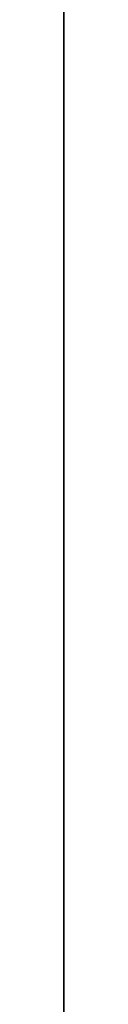
# Model space of a CAD drawing. Units: inches. Extents: x 2083 to 3317, y 1141 to 2115.
# Tile 37 of 256: x 2235.95978 to 2235.95981, y 1477.84234 to 1477.92601. Entities that reach past the tile are written whole.
import ezdxf

# ---------------------------------------------------------------- set-up
doc = ezdxf.new("R2010")
doc.units = ezdxf.units.IN
doc.layers.add('A-ANNO-DIMS', color=2, linetype='Continuous', lineweight=18)
doc.layers.add('A-WALL', color=7, linetype='Continuous', lineweight=35)
doc.layers.add('A-WALL-PATT', color=251, linetype='Continuous', lineweight=13, true_color=0x636466)
doc.styles.get("Standard").update_dxf_attribs({"font": 'arial.ttf'})
doc.dimstyles.new('ISO-25', dxfattribs={"dimtxt": 12, "dimasz": 12, "dimexe": 1.25, "dimexo": 0.625, "dimtad": 1, "dimlunit": 3, "dimtxsty": 'Standard', "dimcen": 2.5, "dimadec": 0, "dimazin": 0, "dimtfac": 1, "dimtmove": 0, "dimatfit": 3, "dimfxl": 1, "dimarcsym": 0})

# ---------------------------------------------------------------- blocks, each defined once
blk = doc.blocks.new('*D30')
at = {"layer": 'A-ANNO-DIMS', "color": 0, "lineweight": -2, "transparency": 16777216}
for p, q in [((2240.017856, 1445.273807), (2240.017856, 1448.045528)), ((2254.329327, 1445.273807), (2254.329327, 1448.045528)), ((2228.017856, 1446.795528), (2216.017856, 1446.795528)), ((2240.017856, 1446.795528), (2254.329327, 1446.795528)), ((2266.329327, 1446.795528), (2413.764866, 1446.795528))]:
    blk.add_line(p, q, dxfattribs=at)
at = {"layer": 'A-ANNO-DIMS', "color": 0, "transparency": 16777216}
for points in [[(2228.017856, 1448.795528), (2228.017856, 1444.795528), (2240.017856, 1446.795528)], [(2266.329327, 1448.795528), (2266.329327, 1444.795528), (2254.329327, 1446.795528)]]:
    blk.add_solid(points, dxfattribs=at)
at = {"layer": 'Defpoints', "color": 0, "transparency": 16777216}
for p in [(2254.329327, 1446.795528), (2240.017856, 1444.648807), (2254.329327, 1444.648807)]:
    blk.add_point(p, dxfattribs=at)
at = {"layer": 'A-ANNO-DIMS', "color": 0, "transparency": 16777216, "insert": (2346.047096, 1453.625167), "char_height": 12, "attachment_point": 5}
blk.add_mtext('WC 1\'-2 1/2" TYP.', dxfattribs=at)
blk = doc.blocks.new('*D31')
at = {"layer": 'A-ANNO-DIMS', "color": 0, "lineweight": -2, "transparency": 16777216}
for p, q in [((2237.871136, 1456.648807), (2237.871136, 1541.915179)), ((2239.392856, 1444.648807), (2236.621136, 1444.648807)), ((2237.871136, 1431.547542), (2237.871136, 1444.648807)), ((2239.392856, 1431.547542), (2236.621136, 1431.547542)), ((2237.871136, 1419.547542), (2237.871136, 1407.547542))]:
    blk.add_line(p, q, dxfattribs=at)
at = {"layer": 'A-ANNO-DIMS', "color": 0, "transparency": 16777216}
for points in [[(2235.871136, 1456.648807), (2239.871136, 1456.648807), (2237.871136, 1444.648807)], [(2235.871136, 1419.547542), (2239.871136, 1419.547542), (2237.871136, 1431.547542)]]:
    blk.add_solid(points, dxfattribs=at)
at = {"layer": 'Defpoints', "color": 0, "transparency": 16777216}
for p in [(2237.871136, 1444.648807), (2240.017856, 1444.648807), (2240.017856, 1431.547542)]:
    blk.add_point(p, dxfattribs=at)
at = {"layer": 'A-ANNO-DIMS', "color": 0, "transparency": 16777216, "insert": (2231.217486, 1505.281993), "char_height": 12, "attachment_point": 5, "rotation": 90}
blk.add_mtext('1\'-1" TYP.', dxfattribs=at)
blk = doc.blocks.new('*D45')
at = {"layer": 'A-ANNO-DIMS', "color": 0, "lineweight": -2, "transparency": 16777216}
for p, q in [((2235.959783, 1478.38636), (2235.959783, 1531.36136)), ((2418.959783, 1478.38636), (2418.959783, 1531.36136)), ((2247.959783, 1530.11136), (2406.959783, 1530.11136))]:
    blk.add_line(p, q, dxfattribs=at)
at = {"layer": 'A-ANNO-DIMS', "color": 0, "transparency": 16777216}
for points in [[(2247.959783, 1532.11136), (2247.959783, 1528.11136), (2235.959783, 1530.11136)], [(2406.959783, 1532.11136), (2406.959783, 1528.11136), (2418.959783, 1530.11136)]]:
    blk.add_solid(points, dxfattribs=at)
at = {"layer": 'Defpoints', "color": 0, "transparency": 16777216}
for p in [(2418.959783, 1530.11136), (2235.959783, 1477.76136), (2418.959783, 1477.76136)]:
    blk.add_point(p, dxfattribs=at)
at = {"layer": 'A-ANNO-DIMS', "color": 0, "transparency": 16777216, "insert": (2327.459783, 1536.867329), "char_height": 12, "attachment_point": 5}
blk.add_mtext('15\'-3"', dxfattribs=at)
blk = doc.blocks.new('*D62')
at = {"layer": 'A-ANNO-DIMS', "color": 0, "lineweight": -2, "transparency": 16777216}
for p, q in [((2235.959783, 1469.38636), (2235.959783, 1522.36136)), ((2379.959783, 1469.38636), (2379.959783, 1522.36136)), ((2247.959783, 1521.11136), (2367.959783, 1521.11136))]:
    blk.add_line(p, q, dxfattribs=at)
at = {"layer": 'A-ANNO-DIMS', "color": 0, "transparency": 16777216}
for points in [[(2247.959783, 1523.11136), (2247.959783, 1519.11136), (2235.959783, 1521.11136)], [(2367.959783, 1523.11136), (2367.959783, 1519.11136), (2379.959783, 1521.11136)]]:
    blk.add_solid(points, dxfattribs=at)
at = {"layer": 'Defpoints', "color": 0, "transparency": 16777216}
for p in [(2379.959783, 1521.11136), (2235.959783, 1468.76136), (2379.959783, 1468.76136)]:
    blk.add_point(p, dxfattribs=at)
at = {"layer": 'A-ANNO-DIMS', "color": 0, "transparency": 16777216, "insert": (2307.959783, 1527.863236), "char_height": 12, "attachment_point": 5}
blk.add_mtext('12\'-0"', dxfattribs=at)

msp = doc.modelspace()

# ---------------------------------------------------------------- hatches: boundary and pattern name
at = {"layer": 'A-WALL-PATT'}
h = msp.add_hatch(color=256, dxfattribs=at)
h.dxf.hatch_style = 1
h.paths.add_polyline_path([(3126.959783, 2020.76136), (2748.959783, 2020.76136), (2604.959783, 2020.76136), (2226.959783, 2020.76136), (2226.959783, 1702.76136), (2466.959783, 1702.76136), (2466.959783, 1582.76136), (2418.959783, 1582.76136), (2418.959783, 1477.76136), (2226.959783, 1477.76136), (2226.959783, 1263.26136), (2544.959783, 1263.26136), (2544.959783, 1411.76136), (2604.959783, 1411.76136), (2685.959783, 1411.76136), (2685.959783, 1420.76136), (2604.959783, 1420.76136), (2604.959783, 1573.76136), (2604.959783, 1702.76136), (2604.959783, 2011.76136), (2748.959783, 2011.76136), (2748.959783, 1702.76136), (2862.959783, 1702.76136), (2862.959783, 1621.76136), (2871.959783, 1621.76136), (2871.959783, 1702.76136), (2883.959783, 1702.76136), (2883.959783, 1706.939459, -0.026459), (2883.959783, 1711.76136), (2757.959783, 1711.76136), (2757.959783, 1807.76136), (2787.959783, 1807.76136), (2787.959783, 1812.26136), (2757.959783, 1812.26136), (2757.959783, 2011.76136), (2877.959783, 2011.76136), (2877.959783, 1812.26136), (2847.959783, 1812.26136), (2847.959783, 1807.76136), (2889.835742, 1807.76136), (2889.835742, 1812.26136), (2882.459783, 1812.26136), (2882.459783, 2011.76136), (3117.959783, 2011.76136), (3117.959783, 1812.26136), (2937.835742, 1812.26136), (2937.835742, 1807.76136), (2995.709783, 1807.76136), (2995.709783, 1796.117666), (3000.209783, 1796.117666), (3000.209783, 1807.76136), (3117.959783, 1807.76136), (3117.959783, 1711.76136), (3000.209783, 1711.76136), (3000.209783, 1760.117666), (2998.572705, 1760.117666, -0.020711), (2995.709783, 1760.117666), (2995.709783, 1711.76136), (2931.959783, 1711.76136), (2931.959783, 1702.76136), (3126.959783, 1702.76136)])
h.paths.add_polyline_path([(2471.459783, 2011.76136), (2471.459783, 1810.01136), (2462.716936, 1810.01136), (2462.716936, 1805.51136), (2505.959783, 1805.51136), (2505.959783, 1810.01136), (2475.959783, 1810.01136), (2475.959783, 2011.76136), (2595.959783, 2011.76136), (2595.959783, 1810.01136), (2565.959783, 1810.01136), (2565.959783, 1805.51136), (2595.959783, 1805.51136), (2595.959783, 1711.76136), (2235.959783, 1711.76136), (2235.959783, 1805.51136), (2353.709783, 1805.51136), (2353.709783, 1796.054162), (2358.209783, 1796.054162), (2358.209783, 1805.51136), (2414.716936, 1805.51136), (2414.716936, 1810.01136), (2235.959783, 1810.01136), (2235.959783, 2011.76136)], flags=16)
h.paths.add_polyline_path([(2270.204734, 1994.610008), (2270.204734, 1970.610008), (2246.204734, 1970.610008), (2246.204734, 1994.610008)], flags=0)
edge = h.paths.add_edge_path(flags=0)
edge.add_ellipse((2332.027391, 1899.798176), major_axis=(-3.042994, 3.042994), ratio=0.16825245, start_angle=-161.332166, end_angle=-156.307114, ccw=False)
edge.add_ellipse((2333.082037, 1898.74353), major_axis=(-1.054646, 1.054646), ratio=0.4535321, start_angle=-123.371019, end_angle=-94.159107)
edge = h.paths.add_edge_path(flags=0)
edge.add_ellipse((2332.027391, 1968.87629), major_axis=(3.042994, 3.042994), ratio=0.16825245, start_angle=18.667834, end_angle=23.692886)
edge.add_spline(control_points=[(2332.925596, 1970.691105), (2332.226768, 1970.3361), (2330.893709, 1969.658905), (2328.41308, 1970.932138), (2327.203934, 1967.748712), (2324.709596, 1969.955589), (2322.532822, 1967.012354), (2320.012846, 1971.295812), (2317.680308, 1968.157845), (2316.040526, 1967.102047), (2315.426904, 1966.809602)], knot_values=[0, 0, 0, 0, 2.267059, 4.324559, 6.685584, 8.878641, 11.121502, 14.300359, 17.755284, 19.732645, 19.732645, 19.732645, 19.732645], degree=3, periodic=0)
edge.add_ellipse((2332.027391, 1968.87629), major_axis=(3.042994, 3.042994), ratio=0.16825245, start_angle=18.667834, end_angle=23.692886, ccw=False)
edge.add_ellipse((2333.082037, 1969.930936), major_axis=(1.054646, 1.054646), ratio=0.4535321, start_angle=56.628981, end_angle=85.840893, ccw=False)
edge = h.paths.add_edge_path(flags=0)
edge.add_spline(control_points=[(2296.428287, 1967.987908), (2293.627804, 1965.336314), (2287.703624, 1959.727094), (2299.74386, 1949.995699), (2294.532591, 1935.668528), (2290.573228, 1920.603512), (2293.394124, 1909.973691), (2296.185407, 1904.966543)], knot_values=[0.099185, 0.099185, 0.099185, 0.099185, 0.345301, 0.619822, 0.982653, 1.386093, 1.810555, 1.810555, 1.810555, 1.810555], degree=3, periodic=0)
edge.add_spline(control_points=[(2296.185407, 1904.966543), (2297.383582, 1902.6193), (2298.000969, 1901.949312), (2298.55297, 1901.468155)], knot_values=[0.006246, 0.006246, 0.006246, 0.006246, 0.055476, 0.055476, 0.055476, 0.055476], degree=3, periodic=0)
edge.add_spline(control_points=[(2298.55297, 1901.468155), (2297.258612, 1900.923224), (2295.225294, 1900.232126), (2293.060229, 1900.614205), (2292.101423, 1900.788415), (2292.089578, 1900.790568)], knot_values=[0.312835, 0.312835, 0.312835, 0.312835, 0.40178, 0.474987, 0.475903, 0.475903, 0.475903, 0.475903], degree=3, periodic=0)
edge.add_arc((2292.793646, 1904.664109), 3.937008, 215.420897, 259.698179, ccw=False)
edge.add_spline(control_points=[(2289.585314, 1902.382304), (2289.476652, 1902.535087), (2289.36848, 1902.688035), (2289.260865, 1902.84117)], knot_values=[0.102872, 0.102872, 0.102872, 0.102872, 0.116896, 0.116896, 0.116896, 0.116896], degree=3, periodic=0)
edge.add_spline(control_points=[(2289.260865, 1902.84117), (2288.686604, 1902.550192), (2287.640048, 1902.019902), (2285.881337, 1901.873954), (2283.852972, 1901.504352), (2281.719987, 1899.710538), (2278.466991, 1899.492942), (2276.157136, 1901.883202), (2272.258953, 1899.804071), (2267.777605, 1901.843183), (2262.243882, 1900.184033), (2257.414927, 1901.782061), (2254.318374, 1900.72612), (2253.178285, 1900.337343)], knot_values=[0, 0, 0, 0, 1.907977, 3.477176, 5.261074, 7.972851, 11.680248, 13.717921, 16.939592, 22.789562, 27.502503, 33.595215, 37.145618, 37.145618, 37.145618, 37.145618], degree=3, periodic=0)
edge.add_line((2253.178285, 1900.337343), (2250.24424, 1902.84117))
edge.add_line((2250.24424, 1902.84117), (2250.24424, 1965.833296))
edge.add_line((2250.24424, 1965.833296), (2253.178285, 1968.337123))
edge.add_spline(control_points=[(2253.178285, 1968.337123), (2254.318374, 1967.948346), (2257.414927, 1966.892405), (2262.243882, 1968.490433), (2267.777605, 1966.831283), (2271.52673, 1968.537217), (2273.875914, 1967.828289), (2274.206701, 1967.727642)], knot_values=[0, 0, 0, 0, 0.09018, 0.244935, 0.364644, 0.513233, 0.537855, 0.537855, 0.537855, 0.537855], degree=3, periodic=0)
edge.add_arc((2274.352887, 1963.793349), 3.937008, 72.051134, 92.127949, ccw=False)
edge.add_arc((2281.296933, 1985.230003), 18.596298, 252.0511336, 288.5657217)
edge.add_arc((2292.316717, 1956.02888), 12.646081, 71.0267879, 113.7782184, ccw=False)
edge = h.paths.add_edge_path(flags=0)
edge.add_spline(control_points=[(2274.899415, 1951.856195), (2275.066156, 1951.616592), (2275.232687, 1951.376588), (2275.397987, 1951.135855)], knot_values=[1.409916, 1.409916, 1.409916, 1.409916, 1.43159, 1.43159, 1.43159, 1.43159], degree=3, periodic=0)
edge.add_spline(control_points=[(2275.397987, 1951.135855), (2275.792106, 1950.561885), (2276.179231, 1949.983774), (2276.545546, 1949.397103)], knot_values=[1.358238, 1.358238, 1.358238, 1.358238, 1.409916, 1.409916, 1.409916, 1.409916], degree=3, periodic=0)
edge.add_line((2276.545546, 1949.397103), (2277.437289, 1947.862185))
edge.add_spline(control_points=[(2277.437289, 1947.862185), (2276.303834, 1945.673115), (2274.639698, 1942.426882), (2274.631615, 1938.0939), (2272.799124, 1930.85155), (2274.356426, 1943.897046), (2275.947681, 1947.923356), (2276.545546, 1949.397103)], knot_values=[0.005632, 0.005632, 0.005632, 0.005632, 0.186014, 0.266002, 0.357087, 0.59639, 0.739732, 0.739732, 0.739732, 0.739732], degree=3, periodic=0)
edge.add_spline(control_points=[(2276.545546, 1949.397103), (2276.179231, 1949.983774), (2275.792106, 1950.561885), (2275.397987, 1951.135855)], knot_values=[1.358238, 1.358238, 1.358238, 1.358238, 1.409916, 1.409916, 1.409916, 1.409916], degree=3, periodic=0)
edge.add_spline(control_points=[(2275.397987, 1951.135855), (2274.9425, 1950.080452), (2274.20776, 1948.025272), (2273.934602, 1944.851477), (2272.468534, 1937.627489), (2273.466216, 1945.696466), (2274.700615, 1951.059472), (2274.899415, 1951.856195)], knot_values=[0.104364, 0.104364, 0.104364, 0.104364, 0.189636, 0.269624, 0.36071, 0.600013, 0.644622, 0.644622, 0.644622, 0.644622], degree=3, periodic=0)
h.paths.add_polyline_path([(2269.167514, 1963.127573, -0.357527), (2268.170633, 1960.97637, -0.092561), (2268.170633, 1939.436325, -0.357527), (2269.167514, 1937.285122, -0.357527), (2267.01631, 1938.282002, -0.164785), (2254.685581, 1938.282002, -0.357527), (2252.534378, 1937.285122, -0.357527), (2253.531259, 1939.436325, -0.092561), (2253.531259, 1960.97637, -0.357527), (2252.534378, 1963.127573, -0.357527), (2254.685581, 1962.130692, -0.164785), (2267.01631, 1962.130692, -0.357527)], flags=0)
h.paths.add_polyline_path([(2248.874068, 1967.8018), (2248.874068, 1957.02771), (2249.457783, 1957.02771), (2249.457783, 1911.646756), (2248.874068, 1911.646756), (2248.874068, 1900.872666), (2246.511863, 1900.872666, 0.197327), (2244.149658, 1902.456873), (2244.149658, 1966.217592, 0.197327), (2246.511863, 1967.8018)], flags=0)
h.paths.add_polyline_path([(2269.167514, 1931.389344, -0.357527), (2268.170633, 1929.238141, -0.092561), (2268.170633, 1907.698096, -0.357527), (2269.167514, 1905.546893, -0.357527), (2267.01631, 1906.543774, -0.164785), (2254.685581, 1906.543774, -0.357527), (2252.534378, 1905.546893, -0.357527), (2253.531259, 1907.698096, -0.092561), (2253.531259, 1929.238141, -0.357527), (2252.534378, 1931.389344, -0.357527), (2254.685581, 1930.392463, -0.164785), (2267.01631, 1930.392463, -0.357527)], flags=0)
edge = h.paths.add_edge_path(flags=0)
edge.add_spline(control_points=[(2276.196858, 1906.723702), (2276.168144, 1909.028928), (2276.114049, 1913.371852), (2270.598417, 1924.924978), (2273.905175, 1919.012779), (2275.921711, 1916.262063), (2275.47457, 1912.402149), (2277.257874, 1910.380621), (2276.696044, 1908.225036), (2276.646218, 1906.813023), (2276.617825, 1906.008407)], knot_values=[0, 0, 0, 0, 8.61026, 16.221274, 18.843057, 23.804898, 27.440828, 29.356102, 31.203478, 33.650687, 33.650687, 33.650687, 33.650687], degree=3, periodic=0)
edge.add_spline(control_points=[(2276.617825, 1906.008407), (2276.623313, 1905.624144), (2276.497738, 1904.628661), (2275.441779, 1903.854725), (2274.937314, 1903.08045), (2274.85908, 1902.84117)], knot_values=[0.156488, 0.156488, 0.156488, 0.156488, 0.184398, 0.231376, 0.250598, 0.250598, 0.250598, 0.250598], degree=3, periodic=0)
edge.add_line((2274.85908, 1902.84117), (2276.50598, 1902.84117))
edge.add_spline(control_points=[(2276.50598, 1902.84117), (2276.788308, 1903.08494), (2277.665071, 1904.125196), (2278.249538, 1904.340738), (2277.653872, 1908.527387), (2278.15567, 1906.227808), (2278.100464, 1905.285948), (2278.846675, 1904.069005), (2277.856785, 1903.414948), (2277.874191, 1902.99105), (2277.903562, 1902.84117)], knot_values=[0.059574, 0.059574, 0.059574, 0.059574, 0.080753, 0.103741, 0.16972, 0.176036, 0.207137, 0.240474, 0.262341, 0.27366, 0.27366, 0.27366, 0.27366], degree=3, periodic=0)
edge.add_line((2277.903562, 1902.84117), (2280.029825, 1902.84117))
edge.add_spline(control_points=[(2280.029825, 1902.84117), (2279.888221, 1903.088398), (2279.499257, 1903.981551), (2280.152284, 1905.939349), (2278.103615, 1909.657757), (2279.762395, 1907.185285), (2280.3279, 1904.874861), (2280.485109, 1903.48959), (2281.463269, 1903.249432), (2281.758343, 1902.936497), (2281.834036, 1902.84117)], knot_values=[0.013856, 0.013856, 0.013856, 0.013856, 0.034874, 0.088867, 0.107879, 0.126738, 0.158714, 0.193757, 0.217487, 0.226722, 0.226722, 0.226722, 0.226722], degree=3, periodic=0)
edge.add_spline(control_points=[(2281.834036, 1902.84117), (2281.787535, 1902.826703), (2281.647022, 1902.782988), (2281.395527, 1902.85949), (2281.088077, 1902.985242), (2280.720683, 1903.060902), (2280.333451, 1903.025726), (2280.124767, 1902.898879), (2280.029825, 1902.84117)], knot_values=[0, 0, 0, 0, 0.14413, 0.435517, 0.749276, 1.153046, 1.548371, 1.878348, 1.878348, 1.878348, 1.878348], degree=3, periodic=0)
edge.add_line((2280.029825, 1902.84117), (2277.903562, 1902.84117))
edge.add_spline(control_points=[(2277.903562, 1902.84117), (2277.892855, 1902.795855), (2277.865396, 1902.679637), (2277.607479, 1902.687483), (2277.27405, 1902.8007), (2276.837921, 1902.619775), (2276.583807, 1902.789261), (2276.50598, 1902.84117)], knot_values=[0, 0, 0, 0, 0.127189, 0.326199, 0.628009, 1.24357, 1.515331, 1.515331, 1.515331, 1.515331], degree=3, periodic=0)
edge.add_line((2276.50598, 1902.84117), (2274.85908, 1902.84117))
edge.add_spline(control_points=[(2274.85908, 1902.84117), (2274.814437, 1902.898587), (2274.72513, 1903.013446), (2274.493477, 1903.118968), (2274.244285, 1902.960539), (2273.937121, 1903.184942), (2273.614039, 1902.983143), (2273.408316, 1902.883045), (2273.322254, 1902.84117)], knot_values=[0, 0, 0, 0, 0.21843, 0.436957, 0.687977, 0.990379, 1.398396, 1.69185, 1.69185, 1.69185, 1.69185], degree=3, periodic=0)
edge.add_spline(control_points=[(2273.322254, 1902.84117), (2273.61674, 1903.445692), (2274.273998, 1904.538253), (2276.027239, 1904.573702), (2276.206963, 1906.583637), (2276.196858, 1906.723702)], knot_values=[0.012227, 0.012227, 0.012227, 0.012227, 0.059472, 0.106218, 0.134458, 0.134458, 0.134458, 0.134458], degree=3, periodic=0)
h.paths.add_polyline_path([(2270.776054, 1897.789828), (2270.776054, 1873.789828), (2246.776054, 1873.789828), (2246.776054, 1897.789828)], flags=0)
h.paths.add_polyline_path([(2353.709783, 1760.005059), (2353.709783, 1760.054162), (2358.209783, 1760.054162, -0.033729)], flags=0)
h.paths.add_polyline_path([(2321.819119, 1737.529186), (2341.995327, 1737.529186, -0.414214), (2343.203273, 1736.321241), (2343.203273, 1721.020596, -0.414214), (2341.995327, 1719.812651), (2321.819119, 1719.812651, -0.414214), (2320.611173, 1721.020596), (2320.611173, 1736.321241, -0.414214)], flags=0)
h.paths.add_polyline_path([(2324.23501, 1736.321241), (2339.579436, 1736.321241, -0.414214), (2341.995327, 1733.905349), (2341.995327, 1725.44973, -0.414214), (2339.579436, 1723.033839), (2333.680588, 1723.033839), (2333.845317, 1722.045467, -0.870646), (2335.425399, 1721.825893, -0.767327), (2333.922694, 1721.423245), (2331.291024, 1721.423245, -0.767327), (2329.788319, 1721.825893, -0.870646), (2331.368401, 1722.045467), (2331.53313, 1723.033839), (2324.23501, 1723.033839, -0.414214), (2321.819119, 1725.44973), (2321.819119, 1733.905349, -0.414214)], flags=0)
h.paths.add_polyline_path([(2570.483789, 1928.615444), (2589.683789, 1928.615444), (2590.168829, 1928.615444), (2590.168829, 1904.993397), (2570.483789, 1904.993397)], flags=0)
h.paths.add_polyline_path([(2574.447324, 1927.263822, -1), (2572.828836, 1927.263822, -1)], flags=0)
h.paths.add_polyline_path([(2573.089867, 1926.940877), (2573.925032, 1927.776042), (2574.147743, 1927.553332), (2573.312577, 1926.718166)], flags=0)
h.paths.add_polyline_path([(2578.779065, 1919.729618, -1), (2571.591663, 1919.729618, -1)], flags=0)
h.paths.add_polyline_path([(2578.385364, 1919.729618, -1), (2571.985364, 1919.729618, -1)], flags=0)
h.paths.add_polyline_path([(2331.595764, 1729.476216, -1), (2333.617954, 1729.476216, -1)], flags=0)
h.paths.add_polyline_path([(2578.034228, 1927.263822, -1), (2576.41574, 1927.263822, -1)], flags=0)
h.paths.add_polyline_path([(2576.688851, 1927.531089), (2576.911562, 1927.753799), (2577.746728, 1926.918634), (2577.524017, 1926.695923)], flags=0)
h.paths.add_polyline_path([(2578.139065, 1909.859539, -1), (2572.231663, 1909.859539, -1)], flags=0)
h.paths.add_polyline_path([(2577.745364, 1909.859539, -1), (2572.625364, 1909.859539, -1)], flags=0)
h.paths.add_polyline_path([(2583.797718, 1927.263822, -1), (2582.179229, 1927.263822, -1)], flags=0)
h.paths.add_polyline_path([(2582.718649, 1927.753799), (2583.553814, 1926.918634), (2583.331103, 1926.695923), (2582.495938, 1927.531089)], flags=0)
h.paths.add_polyline_path([(2582.495938, 1927.531089), (2582.718649, 1927.753799), (2583.553814, 1926.918634), (2583.331103, 1926.695923)], flags=0)
h.paths.add_polyline_path([(2587.739065, 1920.529618, -1), (2581.831663, 1920.529618, -1)], flags=0)
h.paths.add_polyline_path([(2587.345364, 1920.529618, -1), (2582.225364, 1920.529618, -1)], flags=0)
h.paths.add_polyline_path([(2587.384622, 1927.263822, -1), (2585.766133, 1927.263822, -1)], flags=0)
h.paths.add_polyline_path([(2586.081993, 1926.980247), (2586.917158, 1927.815412), (2587.139869, 1927.592702), (2586.304703, 1926.757536)], flags=0)
h.paths.add_polyline_path([(2588.379065, 1910.659539, -1), (2581.191663, 1910.659539, -1)], flags=0)
h.paths.add_polyline_path([(2587.985364, 1910.659539, -1), (2581.585364, 1910.659539, -1)], flags=0)
h.paths.add_polyline_path([(2417.167729, 1729.477895), (2437.343937, 1729.477895, -0.414214), (2438.551883, 1728.26995), (2438.551883, 1712.969306, -0.414214), (2437.343937, 1711.76136), (2417.167729, 1711.76136, -0.414214), (2415.959783, 1712.969306), (2415.959783, 1728.26995, -0.414214)], flags=0)
h.paths.add_polyline_path([(2419.58362, 1728.26995), (2434.928046, 1728.26995, -0.414214), (2437.343937, 1725.854059), (2437.343937, 1717.39844, -0.414214), (2434.928046, 1714.982548), (2429.029199, 1714.982548), (2429.193927, 1713.994176, -0.870646), (2430.774009, 1713.774603, -0.767327), (2429.271304, 1713.371954), (2426.639634, 1713.371954, -0.767327), (2425.136929, 1713.774603, -0.870646), (2426.717011, 1713.994176), (2426.88174, 1714.982548), (2419.58362, 1714.982548, -0.414214), (2417.167729, 1717.39844), (2417.167729, 1725.854059, -0.414214)], flags=0)
h.paths.add_polyline_path([(2419.58362, 1728.26995), (2434.928046, 1728.26995, -0.414214), (2437.343937, 1725.854059), (2437.343937, 1717.39844, -0.414214), (2434.928046, 1714.982548), (2429.029199, 1714.982548), (2428.358118, 1719.009034), (2427.552821, 1719.009034), (2426.88174, 1714.982548), (2419.58362, 1714.982548, -0.414214), (2417.167729, 1717.39844), (2417.167729, 1725.854059, -0.414214)], flags=0)
h.paths.add_polyline_path([(2426.944374, 1721.424925, -1), (2428.966564, 1721.424925, -1)], flags=0)
h.paths.add_polyline_path([(2475.959783, 1702.76136), (2595.959783, 1702.76136), (2595.959783, 1582.76136), (2475.959783, 1582.76136)], flags=16)
h.paths.add_polyline_path([(2427.959783, 1573.76136), (2595.959783, 1573.76136), (2595.959783, 1468.76136), (2595.959783, 1420.76136), (2384.459783, 1420.76136), (2384.459783, 1468.76136), (2427.959783, 1468.76136)], flags=16)
h.paths.add_polyline_path([(2379.959783, 1468.76136), (2379.959783, 1420.76136), (2235.959783, 1420.76136), (2235.959783, 1468.76136)], flags=16)
h.paths.add_polyline_path([(2317.815996, 1466.695767), (2337.992205, 1466.695767, -0.414214), (2339.20015, 1465.487821), (2339.20015, 1450.187177, -0.414214), (2337.992205, 1448.979232), (2317.815996, 1448.979232, -0.414214), (2316.608051, 1450.187177), (2316.608051, 1465.487821, -0.414214)], flags=0)
h.paths.add_polyline_path([(2320.231887, 1465.487821), (2335.576313, 1465.487821, -0.414214), (2337.992205, 1463.07193), (2337.992205, 1454.616311, -0.414214), (2335.576313, 1452.20042), (2329.677466, 1452.20042), (2329.842195, 1451.212047, -0.870646), (2331.422276, 1450.992474, -0.767327), (2329.919571, 1450.589826), (2327.287902, 1450.589826, -0.767327), (2325.785197, 1450.992474, -0.870646), (2327.365278, 1451.212047), (2327.530007, 1452.20042), (2320.231887, 1452.20042, -0.414214), (2317.815996, 1454.616311), (2317.815996, 1463.07193, -0.414214)], flags=0)
h.paths.add_polyline_path([(2320.231887, 1465.487821), (2335.576313, 1465.487821, -0.414214), (2337.992205, 1463.07193), (2337.992205, 1454.616311, -0.414214), (2335.576313, 1452.20042), (2329.677466, 1452.20042), (2329.006385, 1456.226905), (2328.201088, 1456.226905), (2327.530007, 1452.20042), (2320.231887, 1452.20042, -0.414214), (2317.815996, 1454.616311), (2317.815996, 1463.07193, -0.414214)], flags=0)
h.paths.add_polyline_path([(2327.592641, 1458.642796, -1), (2329.614832, 1458.642796, -1)], flags=0)
h.paths.add_polyline_path([(2244.411744, 1433.340453), (2241.920945, 1433.340453, -0.414214), (2240.017856, 1435.243542), (2240.017856, 1440.952808, -0.414211), (2241.920925, 1442.855897), (2244.411744, 1442.855897, -1.976472)], flags=0)
h.paths.add_polyline_path([(2245.356888, 1434.397536, -0.414214), (2245.356888, 1441.798814, -2.144098)], flags=0)
h.paths.add_polyline_path([(2535.959783, 1416.26136), (2535.959783, 1272.26136), (2235.959783, 1272.26136), (2235.959783, 1416.26136)], flags=16)
h.paths.add_polyline_path([(2260.119561, 1384.292841), (2260.119561, 1362.038649), (2237.865369, 1362.038649), (2237.865369, 1384.292841)], flags=0)
edge = h.paths.add_edge_path(flags=0)
edge.add_line((2318.251847, 1362.093298), (2318.145797, 1362.000973))
edge.add_ellipse((2317.445116, 1360.431044), major_axis=(2.82164, 2.82164), ratio=0.16825245, start_angle=18.667834, end_angle=20.948127, ccw=False)
edge.add_ellipse((2318.423045, 1361.408974), major_axis=(0.977929, 0.977929), ratio=0.4535321, start_angle=56.628981, end_angle=70.226201, ccw=False)
edge = h.paths.add_edge_path(flags=0)
edge.add_line((2319.10737, 1295.571078), (2319.015044, 1295.677128))
edge.add_ellipse((2317.445116, 1296.377809), major_axis=(-2.82164, 2.82164), ratio=0.16825245, start_angle=-161.332166, end_angle=-159.051873, ccw=False)
edge.add_ellipse((2318.423045, 1295.39988), major_axis=(-0.977929, 0.977929), ratio=0.4535321, start_angle=-123.371019, end_angle=-109.773799)
edge = h.paths.add_edge_path(flags=0)
edge.add_spline(control_points=[(2284.210349, 1301.170219), (2284.580688, 1300.444719), (2284.891189, 1299.892024), (2285.159553, 1299.461018)], knot_values=[0.039066, 0.039066, 0.039066, 0.039066, 0.055476, 0.055476, 0.055476, 0.055476], degree=3, periodic=0)
edge.add_line((2285.159553, 1299.461018), (2284.210349, 1301.170219))
edge = h.paths.add_edge_path(flags=0)
edge.add_line((2280.412458, 1297.298013), (2283.369991, 1297.036122))
edge.add_line((2283.369991, 1297.036122), (2286.40569, 1297.92631))
edge.add_spline(control_points=[(2286.40569, 1297.92631), (2285.305487, 1297.463119), (2284.344777, 1297.129151), (2283.369991, 1297.036122)], knot_values=[0.394369, 0.394369, 0.394369, 0.394369, 0.475903, 0.475903, 0.475903, 0.475903], degree=3, periodic=0)
edge.add_spline(control_points=[(2283.369991, 1297.036122), (2283.28139, 1297.027666), (2282.316289, 1296.957336), (2281.312502, 1297.134479), (2280.423441, 1297.296016), (2280.412458, 1297.298013)], knot_values=[0.312835, 0.312835, 0.312835, 0.312835, 0.320246, 0.393453, 0.394369, 0.394369, 0.394369, 0.394369], degree=3, periodic=0)
edge = h.paths.add_edge_path(flags=0)
edge.add_line((2284.435561, 1359.607285), (2280.446291, 1355.328047))
edge.add_line((2280.446291, 1355.328047), (2279.579987, 1351.017754))
edge.add_line((2279.579987, 1351.017754), (2282.412974, 1346.580433))
edge.add_spline(control_points=[(2282.412974, 1346.580433), (2283.153331, 1345.589236), (2284.252896, 1344.028897), (2284.801037, 1342.387167), (2284.935162, 1341.805544)], knot_values=[1.240098, 1.240098, 1.240098, 1.240098, 1.332892, 1.382712, 1.382712, 1.382712, 1.382712], degree=3, periodic=0)
edge.add_spline(control_points=[(2284.935162, 1341.805544), (2285.319108, 1340.1406), (2285.233029, 1338.409204), (2284.909938, 1336.654122)], knot_values=[1.097484, 1.097484, 1.097484, 1.097484, 1.240098, 1.240098, 1.240098, 1.240098], degree=3, periodic=0)
edge.add_spline(control_points=[(2284.909938, 1336.654122), (2284.586848, 1334.89904), (2284.026745, 1333.120272), (2283.462644, 1331.360585)], knot_values=[0.95487, 0.95487, 0.95487, 0.95487, 1.097484, 1.097484, 1.097484, 1.097484], degree=3, periodic=0)
edge.add_line((2283.462644, 1331.360585), (2281.890376, 1326.153357))
edge.add_line((2281.890376, 1326.153357), (2280.756259, 1321.056089))
edge.add_line((2280.756259, 1321.056089), (2280.299205, 1316.001977))
edge.add_line((2280.299205, 1316.001977), (2280.715933, 1310.950068))
edge.add_line((2280.715933, 1310.950068), (2282.028094, 1305.972137))
edge.add_line((2282.028094, 1305.972137), (2284.210349, 1301.170219))
edge.add_spline(control_points=[(2284.210349, 1301.170219), (2283.340731, 1302.730185), (2282.611904, 1304.336493), (2282.028094, 1305.972137)], knot_values=[0.099185, 0.099185, 0.099185, 0.099185, 0.241799, 0.241799, 0.241799, 0.241799], degree=3, periodic=0)
edge.add_spline(control_points=[(2282.028094, 1305.972137), (2281.444283, 1307.60778), (2281.005489, 1309.272759), (2280.715933, 1310.950068)], knot_values=[0.241799, 0.241799, 0.241799, 0.241799, 0.384413, 0.384413, 0.384413, 0.384413], degree=3, periodic=0)
edge.add_spline(control_points=[(2280.715933, 1310.950068), (2280.433241, 1312.587613), (2280.289386, 1314.276959), (2280.298894, 1315.962032), (2280.299205, 1316.001977)], knot_values=[0.384413, 0.384413, 0.384413, 0.384413, 0.523647, 0.527028, 0.527028, 0.527028, 0.527028], degree=3, periodic=0)
edge.add_spline(control_points=[(2280.299205, 1316.001977), (2280.312326, 1317.686955), (2280.477871, 1319.367926), (2280.756259, 1321.056089)], knot_values=[0.527028, 0.527028, 0.527028, 0.527028, 0.669642, 0.669642, 0.669642, 0.669642], degree=3, periodic=0)
edge.add_spline(control_points=[(2280.756259, 1321.056089), (2281.034648, 1322.744252), (2281.42588, 1324.439608), (2281.890376, 1326.153357)], knot_values=[0.669642, 0.669642, 0.669642, 0.669642, 0.812256, 0.812256, 0.812256, 0.812256], degree=3, periodic=0)
edge.add_spline(control_points=[(2281.890376, 1326.153357), (2282.264383, 1327.533251), (2282.78787, 1329.26181), (2283.352751, 1331.01778), (2283.462644, 1331.360585)], knot_values=[0.812256, 0.812256, 0.812256, 0.812256, 0.927087, 0.95487, 0.95487, 0.95487, 0.95487], degree=3, periodic=0)
edge.add_line((2283.462644, 1331.360585), (2284.909938, 1336.654122))
edge.add_line((2284.909938, 1336.654122), (2284.935162, 1341.805544))
edge.add_line((2284.935162, 1341.805544), (2282.412974, 1346.580433))
edge.add_spline(control_points=[(2282.412974, 1346.580433), (2281.275127, 1348.103792), (2280.078447, 1349.570318), (2279.579987, 1351.017754)], knot_values=[1.382712, 1.382712, 1.382712, 1.382712, 1.525326, 1.525326, 1.525326, 1.525326], degree=3, periodic=0)
edge.add_spline(control_points=[(2279.579987, 1351.017754), (2279.443282, 1351.414721), (2279.136312, 1352.856922), (2279.73519, 1354.290385), (2280.446291, 1355.328047)], knot_values=[1.525326, 1.525326, 1.525326, 1.525326, 1.564439, 1.667941, 1.667941, 1.667941, 1.667941], degree=3, periodic=0)
edge.add_spline(control_points=[(2280.446291, 1355.328047), (2281.426113, 1356.757835), (2282.930837, 1358.18256), (2284.435561, 1359.607285)], knot_values=[1.667941, 1.667941, 1.667941, 1.667941, 1.810555, 1.810555, 1.810555, 1.810555], degree=3, periodic=0)
edge.add_arc((2280.623075, 1348.518181), 11.72618, 71.0267879, 113.7782184)
edge.add_arc((2270.404892, 1375.595156), 17.243567, 252.0511336, 288.5657217, ccw=False)
edge.add_arc((2263.965969, 1355.717847), 3.650622, 72.051134, 92.127949)
edge.add_arc((2263.965969, 1355.717847), 3.650622, 92.127949, 177.98513)
edge.add_spline(control_points=[(2260.317604, 1355.846199), (2260.260417, 1354.220668), (2260.551278, 1350.186547), (2262.999344, 1346.766251), (2264.472741, 1344.649024)], knot_values=[1.43159, 1.43159, 1.43159, 1.43159, 1.564144, 1.770695, 1.770695, 1.770695, 1.770695], degree=3, periodic=0)
edge.add_line((2264.472741, 1344.649024), (2264.93559, 1343.98253))
edge.add_spline(control_points=[(2263.801044, 1340.248105), (2263.843238, 1340.514088), (2264.067244, 1341.756465), (2264.512693, 1343.002453), (2264.935047, 1343.981083)], knot_values=[0.53657, 0.53657, 0.53657, 0.53657, 0.559349, 0.644622, 0.644622, 0.644622, 0.644622], degree=3, periodic=0)
edge.add_spline(control_points=[(2264.935047, 1343.981083), (2265.117771, 1343.714975), (2265.298875, 1343.447906), (2265.476756, 1343.179365)], knot_values=[1.384077, 1.384077, 1.384077, 1.384077, 1.409916, 1.409916, 1.409916, 1.409916], degree=3, periodic=0)
edge.add_spline(control_points=[(2265.476756, 1343.179365), (2265.654637, 1342.910823), (2265.829296, 1342.64081), (2265.99913, 1342.368812)], knot_values=[1.358238, 1.358238, 1.358238, 1.358238, 1.384077, 1.384077, 1.384077, 1.384077], degree=3, periodic=0)
edge.add_line((2265.99913, 1342.368812), (2266.826006, 1340.945547))
edge.add_spline(control_points=[(2266.826006, 1340.945547), (2268.894401, 1337.089691), (2271.398173, 1325.843001), (2270.516164, 1310.568557), (2275.919376, 1301.860609), (2277.789511, 1299.19945)], knot_values=[0.116896, 0.116896, 0.116896, 0.116896, 0.472987, 1.050969, 1.313793, 1.313793, 1.313793, 1.313793], degree=3, periodic=0)
edge.add_spline(control_points=[(2277.789511, 1299.19945), (2277.839405, 1299.128452), (2277.889428, 1299.057498), (2277.939572, 1298.986584)], knot_values=[0.109884, 0.109884, 0.109884, 0.109884, 0.116896, 0.116896, 0.116896, 0.116896], degree=3, periodic=0)
edge.add_line((2277.939572, 1298.986584), (2277.788849, 1299.199114))
edge.add_spline(control_points=[(2277.788849, 1299.199114), (2277.256582, 1298.929414), (2276.28635, 1298.437902), (2275.039352, 1298.334419), (2274.38333, 1298.238895), (2274.215254, 1298.209338)], knot_values=[33.12187, 33.12187, 33.12187, 33.12187, 35.029056, 36.598255, 37.144827, 37.144827, 37.144827, 37.144827], degree=3, periodic=0)
edge.add_line((2274.215254, 1298.209338), (2273.073147, 1297.892961))
edge.add_spline(control_points=[(2273.073147, 1297.892961), (2272.322936, 1297.579784), (2271.039151, 1296.510508), (2269.248395, 1296.226062), (2268.4231, 1296.374654)], knot_values=[26.532584, 26.532584, 26.532584, 26.532584, 29.198919, 31.839101, 31.839101, 31.839101, 31.839101], degree=3, periodic=0)
edge.add_line((2268.4231, 1296.374654), (2263.878501, 1297.457534))
edge.add_spline(control_points=[(2263.878501, 1297.457534), (2263.556077, 1297.359435), (2261.860306, 1296.838694), (2260.23878, 1297.282407), (2258.933454, 1297.516461)], knot_values=[15.919551, 15.919551, 15.919551, 15.919551, 16.939592, 21.226067, 21.226067, 21.226067, 21.226067], degree=3, periodic=0)
edge.add_line((2258.933454, 1297.516461), (2254.055233, 1297.32901))
edge.add_spline(control_points=[(2254.055233, 1297.32901), (2253.755525, 1297.295815), (2252.113683, 1297.165174), (2250.461869, 1297.544221), (2249.129686, 1297.667882)], knot_values=[5.306517, 5.306517, 5.306517, 5.306517, 6.276435, 10.613034, 10.613034, 10.613034, 10.613034], degree=3, periodic=0)
edge.add_line((2249.129686, 1297.667882), (2244.33165, 1296.877756))
edge.add_line((2244.33165, 1296.877756), (2241.611033, 1299.19945))
edge.add_line((2241.611033, 1299.19945), (2241.611033, 1357.609404))
edge.add_line((2241.611033, 1357.609404), (2244.33165, 1359.931097))
edge.add_line((2244.33165, 1359.931097), (2252.728823, 1359.542692))
edge.add_spline(control_points=[(2252.728823, 1359.542692), (2252.870939, 1359.54644), (2253.30574, 1359.548172), (2253.739845, 1359.514274), (2254.031742, 1359.482426)], knot_values=[0.233291, 0.233291, 0.233291, 0.233291, 0.244935, 0.268927, 0.268927, 0.268927, 0.268927], degree=3, periodic=0)
edge.add_line((2254.031742, 1359.482426), (2259.58719, 1359.41639))
edge.add_spline(control_points=[(2259.58719, 1359.41639), (2260.677068, 1359.628503), (2262.073197, 1359.897003), (2263.523692, 1359.459278), (2263.830417, 1359.365952)], knot_values=[0.422516, 0.422516, 0.422516, 0.422516, 0.513233, 0.537855, 0.537855, 0.537855, 0.537855], degree=3, periodic=0)
edge.add_arc((2263.965969, 1355.717847), 3.650622, 72.051134, 92.127949, ccw=False)
edge.add_arc((2270.404892, 1375.595156), 17.243567, 252.0511336, 288.5657217)
edge.add_arc((2280.623075, 1348.518181), 11.72618, 71.0267879, 113.7782184, ccw=False)
h.paths.add_polyline_path([(2240.34053, 1359.434715), (2240.34053, 1349.444353), (2240.881785, 1349.444353), (2240.881785, 1307.3645), (2240.34053, 1307.3645), (2240.34053, 1297.374138), (2238.150157, 1297.374138, 0.197327), (2235.959783, 1298.843108), (2235.959783, 1357.965746, 0.197327), (2238.150157, 1359.434715)], flags=0)
h.paths.add_polyline_path([(2259.15779, 1355.1005, -0.357527), (2258.233425, 1353.10578, -0.092561), (2258.233425, 1333.132601, -0.357527), (2259.15779, 1331.13788, -0.357527), (2257.16307, 1332.062246, -0.164785), (2245.729302, 1332.062246, -0.357527), (2243.734582, 1331.13788, -0.357527), (2244.658947, 1333.132601, -0.092561), (2244.658947, 1353.10578, -0.357527), (2243.734582, 1355.1005, -0.357527), (2245.729302, 1354.176135, -0.164785), (2257.16307, 1354.176135, -0.357527)], flags=0)
edge = h.paths.add_edge_path(flags=0)
edge.add_line((2265.99913, 1342.368812), (2266.826006, 1340.945547))
edge.add_line((2266.826006, 1340.945547), (2265.307557, 1337.814066))
edge.add_line((2265.307557, 1337.814066), (2264.358232, 1334.652939))
edge.add_line((2264.358232, 1334.652939), (2264.262012, 1333.799705))
edge.add_spline(control_points=[(2264.262012, 1333.799705), (2264.208357, 1333.187055), (2264.16206, 1332.365525), (2264.007144, 1331.413933), (2263.969049, 1331.201834)], knot_values=[0.464444, 0.464444, 0.464444, 0.464444, 0.516691, 0.531608, 0.531608, 0.531608, 0.531608], degree=3, periodic=0)
edge.add_spline(control_points=[(2263.969049, 1331.201834), (2263.774535, 1330.118873), (2263.42437, 1328.790839), (2263.25742, 1328.530652), (2263.234028, 1328.514612)], knot_values=[0.372682, 0.372682, 0.372682, 0.372682, 0.44885, 0.464444, 0.464444, 0.464444, 0.464444], degree=3, periodic=0)
edge.add_spline(control_points=[(2263.234028, 1328.514612), (2263.096382, 1328.420227), (2263.13117, 1329.301477), (2263.274953, 1330.615749)], knot_values=[0.280919, 0.280919, 0.280919, 0.280919, 0.372682, 0.372682, 0.372682, 0.372682], degree=3, periodic=0)
edge.add_spline(control_points=[(2263.274953, 1330.615749), (2263.418736, 1331.930022), (2263.671515, 1333.677318), (2263.969852, 1335.315027)], knot_values=[0.189157, 0.189157, 0.189157, 0.189157, 0.280919, 0.280919, 0.280919, 0.280919], degree=3, periodic=0)
edge.add_spline(control_points=[(2263.969852, 1335.315027), (2264.100496, 1336.032192), (2264.418783, 1337.621911), (2264.754848, 1338.86443), (2264.947419, 1339.491124)], knot_values=[0.097394, 0.097394, 0.097394, 0.097394, 0.137578, 0.189157, 0.189157, 0.189157, 0.189157], degree=3, periodic=0)
edge.add_spline(control_points=[(2264.947419, 1339.491124), (2265.290017, 1340.606055), (2265.644238, 1341.493996), (2265.99913, 1342.368812)], knot_values=[0.005632, 0.005632, 0.005632, 0.005632, 0.097394, 0.097394, 0.097394, 0.097394], degree=3, periodic=0)
h.paths.add_polyline_path([(2259.15779, 1325.670973, -0.357527), (2258.233425, 1323.676253, -0.092561), (2258.233425, 1303.703073, -0.357527), (2259.15779, 1301.708353, -0.357527), (2257.16307, 1302.632719, -0.164785), (2245.729302, 1302.632719, -0.357527), (2243.734582, 1301.708353, -0.357527), (2244.658947, 1303.703073, -0.092561), (2244.658947, 1323.676253, -0.357527), (2243.734582, 1325.670973, -0.357527), (2245.729302, 1324.746608, -0.164785), (2257.16307, 1324.746608, -0.357527)], flags=0)
edge = h.paths.add_edge_path(flags=0)
edge.add_spline(control_points=[(2261.708938, 1317.311421), (2261.679482, 1317.41758), (2261.761858, 1317.388535), (2262.490736, 1316.089873), (2262.962185, 1315.300897)], knot_values=[14.955861, 14.955861, 14.955861, 14.955861, 16.221274, 18.694826, 18.694826, 18.694826, 18.694826], degree=3, periodic=0)
edge.add_spline(control_points=[(2262.962185, 1315.300897), (2262.990437, 1315.253617), (2263.702096, 1314.067376), (2264.348983, 1313.127153), (2264.730054, 1312.164154)], knot_values=[18.694826, 18.694826, 18.694826, 18.694826, 18.843057, 22.433791, 22.433791, 22.433791, 22.433791], degree=3, periodic=0)
edge.add_spline(control_points=[(2264.730054, 1312.164154), (2264.875565, 1311.796437), (2265.176873, 1310.769807), (2265.143069, 1309.559262), (2265.247736, 1308.824193)], knot_values=[22.433791, 22.433791, 22.433791, 22.433791, 23.804898, 26.172756, 26.172756, 26.172756, 26.172756], degree=3, periodic=0)
edge.add_line((2265.247736, 1308.824193), (2265.850774, 1307.171888))
edge.add_spline(control_points=[(2265.850774, 1307.171888), (2266.065025, 1306.821678), (2266.384387, 1306.332246), (2266.4244, 1305.780549), (2266.420369, 1305.611216)], knot_values=[28.062562, 28.062562, 28.062562, 28.062562, 29.356102, 29.911721, 29.911721, 29.911721, 29.911721], degree=3, periodic=0)
edge.add_spline(control_points=[(2266.420369, 1305.611216), (2266.416116, 1305.43259), (2266.393999, 1305.249998), (2266.364777, 1305.065857)], knot_values=[29.911721, 29.911721, 29.911721, 29.911721, 30.497837, 30.497837, 30.497837, 30.497837], degree=3, periodic=0)
edge.add_line((2266.364777, 1305.065857), (2266.066151, 1302.136295))
edge.add_spline(control_points=[(2266.066151, 1302.136295), (2266.07124, 1301.779984), (2265.998076, 1301.199985), (2265.663266, 1300.758961), (2265.508908, 1300.585882)], knot_values=[0.156488, 0.156488, 0.156488, 0.156488, 0.184398, 0.203543, 0.203543, 0.203543, 0.203543], degree=3, periodic=0)
edge.add_line((2265.508908, 1300.585882), (2264.435341, 1299.19945))
edge.add_line((2264.435341, 1299.19945), (2265.962442, 1299.19945))
edge.add_line((2265.962442, 1299.19945), (2267.33599, 1301.175276))
edge.add_line((2267.33599, 1301.175276), (2267.311667, 1301.986237))
edge.add_spline(control_points=[(2267.311667, 1301.986237), (2267.261111, 1302.862396), (2267.160212, 1303.737132), (2267.271486, 1303.325896)], knot_values=[0.126229, 0.126229, 0.126229, 0.126229, 0.166617, 0.166617, 0.166617, 0.166617], degree=3, periodic=0)
edge.add_spline(control_points=[(2267.271486, 1303.325896), (2267.280035, 1303.294305), (2267.309785, 1303.175366), (2267.37345, 1302.883608), (2267.406123, 1302.682829), (2267.417926, 1302.601025)], knot_values=[0.166617, 0.166617, 0.166617, 0.166617, 0.16972, 0.176036, 0.180765, 0.180765, 0.180765, 0.180765], degree=3, periodic=0)
edge.add_spline(control_points=[(2267.743891, 1300.987505), (2267.687583, 1301.150943), (2267.48052, 1301.656664), (2267.483751, 1302.144788), (2267.417926, 1302.601025)], knot_values=[0.180765, 0.180765, 0.180765, 0.180765, 0.193767, 0.220139, 0.220139, 0.220139, 0.220139], degree=3, periodic=0)
edge.add_line((2267.417926, 1302.601025), (2267.743891, 1300.987505))
edge.add_spline(control_points=[(2267.743891, 1300.987505), (2267.831961, 1300.731878), (2267.932021, 1300.309904), (2267.554841, 1299.974518), (2267.429366, 1299.829207)], knot_values=[0.220139, 0.220139, 0.220139, 0.220139, 0.240474, 0.25489, 0.25489, 0.25489, 0.25489], degree=3, periodic=0)
edge.add_line((2267.429366, 1299.829207), (2267.258361, 1299.19945))
edge.add_line((2267.258361, 1299.19945), (2269.229956, 1299.19945))
edge.add_spline(control_points=[(2269.229956, 1299.19945), (2269.098653, 1299.428694), (2268.842774, 1300.016251), (2269.011575, 1300.915923), (2268.946796, 1301.66074)], knot_values=[0.013856, 0.013856, 0.013856, 0.013856, 0.034874, 0.067073, 0.067073, 0.067073, 0.067073], degree=3, periodic=0)
edge.add_line((2268.946796, 1301.66074), (2268.431582, 1303.603109))
edge.add_spline(control_points=[(2268.431582, 1303.603109), (2268.175596, 1304.192375), (2267.596214, 1305.251298), (2268.040698, 1304.62321), (2268.251394, 1304.282421)], knot_values=[0.090155, 0.090155, 0.090155, 0.090155, 0.107879, 0.120289, 0.120289, 0.120289, 0.120289], degree=3, periodic=0)
edge.add_spline(control_points=[(2268.251394, 1304.282421), (2268.360882, 1304.105329), (2269.057753, 1302.917983), (2269.382691, 1301.590419), (2269.521405, 1300.775931), (2269.57522, 1300.555784)], knot_values=[0.120289, 0.120289, 0.120289, 0.120289, 0.126738, 0.158714, 0.173506, 0.173506, 0.173506, 0.173506], degree=3, periodic=0)
edge.add_line((2269.57522, 1300.555784), (2270.685798, 1299.421258))
edge.add_spline(control_points=[(2270.685798, 1299.421258), (2270.767221, 1299.357251), (2270.837852, 1299.281401), (2270.902925, 1299.19945)], knot_values=[0.21816, 0.21816, 0.21816, 0.21816, 0.226722, 0.226722, 0.226722, 0.226722], degree=3, periodic=0)
edge.add_line((2270.937201, 1299.192913), (2270.902925, 1299.19945))
edge.add_spline(control_points=[(2270.902925, 1299.19945), (2270.859806, 1299.186035), (2270.729515, 1299.1455), (2270.496314, 1299.216437), (2270.271661, 1299.308323), (2270.121017, 1299.347961), (2270.063339, 1299.359557)], knot_values=[0.939174, 0.939174, 0.939174, 0.939174, 1.083304, 1.374691, 1.68845, 1.878348, 1.878348, 1.878348, 1.878348], degree=3, periodic=0)
edge.add_line((2270.063339, 1299.359557), (2269.229956, 1299.19945))
edge.add_line((2269.229956, 1299.19945), (2267.258361, 1299.19945))
edge.add_spline(control_points=[(2267.258361, 1299.19945), (2267.248433, 1299.157431), (2267.222971, 1299.049667), (2266.983816, 1299.056942), (2266.80921, 1299.11623), (2266.676905, 1299.109091), (2266.636531, 1299.104815)], knot_values=[0.757665, 0.757665, 0.757665, 0.757665, 0.884854, 1.083864, 1.385675, 1.515331, 1.515331, 1.515331, 1.515331], degree=3, periodic=0)
edge.add_spline(control_points=[(2266.636531, 1299.104815), (2266.485225, 1299.088788), (2266.235807, 1299.017123), (2266.034608, 1299.151317), (2265.962442, 1299.19945)], knot_values=[0, 0, 0, 0, 0.485905, 0.757665, 0.757665, 0.757665, 0.757665], degree=3, periodic=0)
edge.add_line((2265.962442, 1299.19945), (2264.435341, 1299.19945))
edge.add_line((2264.435341, 1299.19945), (2263.858444, 1299.367118))
edge.add_spline(control_points=[(2263.858444, 1299.367118), (2263.818943, 1299.370905), (2263.779528, 1299.385721), (2263.740131, 1299.401504)], knot_values=[0.845925, 0.845925, 0.845925, 0.845925, 0.978627, 0.978627, 0.978627, 0.978627], degree=3, periodic=0)
edge.add_line((2263.721786, 1299.396425), (2263.010306, 1299.19945))
edge.add_spline(control_points=[(2263.010306, 1299.19945), (2263.245794, 1299.682859), (2263.506032, 1300.128107), (2263.873494, 1300.408028)], knot_values=[0.012227, 0.012227, 0.012227, 0.012227, 0.052971, 0.052971, 0.052971, 0.052971], degree=3, periodic=0)
edge.add_spline(control_points=[(2263.873494, 1300.408028), (2263.932131, 1300.452695), (2264.084243, 1300.552979), (2264.255189, 1300.624223), (2264.359686, 1300.664747)], knot_values=[0.052971, 0.052971, 0.052971, 0.052971, 0.059472, 0.069086, 0.069086, 0.069086, 0.069086], degree=3, periodic=0)
edge.add_line((2264.359686, 1300.664747), (2265.1419, 1301.077774))
edge.add_line((2265.1419, 1301.077774), (2265.675806, 1302.799558))
edge.add_line((2265.675806, 1302.799558), (2265.5407, 1305.704066))
edge.add_line((2265.5407, 1305.704066), (2264.803073, 1309.327724))
edge.add_line((2264.803073, 1309.327724), (2263.040535, 1314.091791))
edge.add_spline(control_points=[(2263.040535, 1314.091791), (2262.383572, 1315.671438), (2261.795972, 1316.997749), (2261.708938, 1317.311421)], knot_values=[11.216896, 11.216896, 11.216896, 11.216896, 14.955861, 14.955861, 14.955861, 14.955861], degree=3, periodic=0)
h.paths.add_polyline_path([(2871.959783, 1416.26136), (2895.910047, 1416.26136), (2895.910047, 1420.76136), (2871.959783, 1420.76136), (2871.959783, 1501.76136), (2862.959783, 1501.76136), (2862.959783, 1420.76136), (2805.959783, 1420.76136), (2805.959783, 1411.76136), (2862.959783, 1411.76136), (2862.959783, 1263.26136), (3126.959783, 1263.26136), (3126.959783, 1411.76136), (3126.959783, 1486.76136), (2943.959783, 1486.76136), (2943.959783, 1477.76136), (2967.860311, 1477.76136), (2967.860311, 1420.76136), (2943.910047, 1420.76136), (2943.910047, 1416.26136), (3117.959783, 1416.26136), (3117.959783, 1420.76136), (2972.360311, 1420.76136), (2972.360311, 1477.76136), (3117.959783, 1477.76136), (3117.959783, 1420.76136), (3117.959783, 1272.26136), (2871.959783, 1272.26136)], flags=0)
h.paths.add_polyline_path([(2457.125626, 1485.942505), (2527.602651, 1485.942505), (2527.602651, 1537.635702), (2457.125626, 1537.635702)], flags=8)
h.paths.add_polyline_path([(2481.005058, 1609.981804), (2590.765818, 1609.981804), (2590.765818, 1682.003362), (2481.005058, 1682.003362)], flags=8)
h.paths.add_polyline_path([(2483.085022, 1729.126784), (2553.562048, 1729.126784), (2553.562048, 1780.81998), (2483.085022, 1780.81998)], flags=8)

# ---------------------------------------------------------------- linework, layer by layer
at = {"layer": 'A-WALL'}
msp.add_line((2235.959783, 1702.76136), (2235.959783, 1477.76136), dxfattribs=at)
msp.add_line((2235.959783, 1702.76136), (2235.959783, 1477.76136), dxfattribs=at)

# ---------------------------------------------------------------- dimensions: what is measured, and where the dimension line sits
at = {"layer": 'A-ANNO-DIMS'}
for base, p1, p2, picture, middle in [((2418.959783, 1530.11136), (2235.959783, 1477.76136), (2418.959783, 1477.76136), '*D45', (2327.459783, 1536.867329)), ((2379.959783, 1521.11136), (2235.959783, 1468.76136), (2379.959783, 1468.76136), '*D62', (2307.959783, 1527.863236))]:
    dim = msp.add_linear_dim(base=base, p1=p1, p2=p2, dimstyle='ISO-25', override={"dimdec": 1, "dimlfac": 1, "dimrnd": 0, "dimzin": 1, "dimdsep": 46, "dimlunit": 4, "dimfrac": 2}, dxfattribs=at)
    dim.commit()
    dim.dimension.update_dxf_attribs({"geometry": picture, "text_midpoint": middle})
dim = msp.add_linear_dim(base=(2237.871136, 1444.648807), p1=(2240.017856, 1431.547542), p2=(2240.017856, 1444.648807), angle=90, text='<> TYP.', dimstyle='ISO-25', override={"dimdec": 1, "dimlfac": 1, "dimrnd": 0, "dimzin": 1, "dimdsep": 46, "dimlunit": 4, "dimfrac": 2}, dxfattribs=at)
dim.commit()
dim.dimension.update_dxf_attribs({"geometry": '*D31', "text_midpoint": (2231.217486, 1505.281993)})
dim = msp.add_linear_dim(base=(2254.329327, 1446.795528), p1=(2240.017856, 1444.648807), p2=(2254.329327, 1444.648807), text='WC <> TYP.', dimstyle='ISO-25', override={"dimdec": 1, "dimlfac": 1, "dimrnd": 0, "dimzin": 1, "dimdsep": 46, "dimlunit": 4, "dimfrac": 2}, dxfattribs=at)
dim.commit()
dim.dimension.update_dxf_attribs({"geometry": '*D30', "text_midpoint": (2346.047096, 1453.625167)})

doc.saveas('drawing.dxf')
